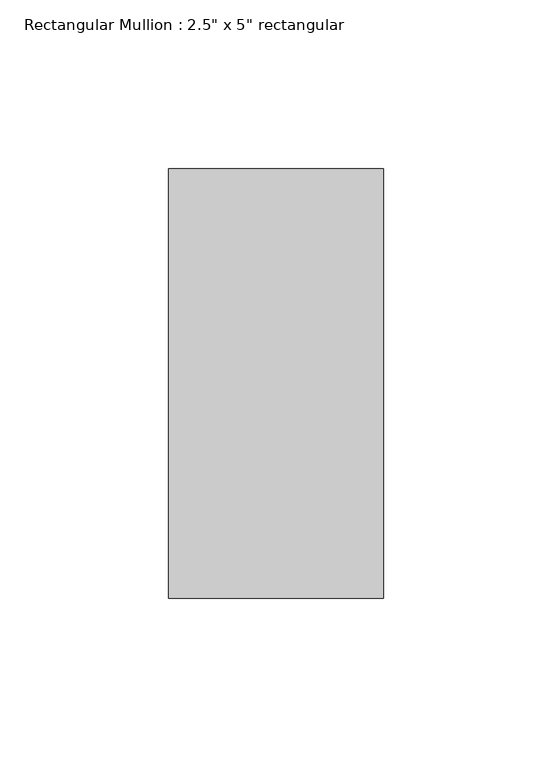
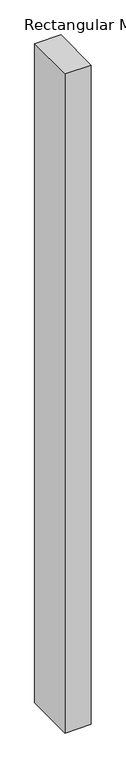
"""IFC4 building model written with IfcOpenShell, lengths in millimetres: member geometry."""

from ifc_helpers import new_model, si_unit, frame, origin, place, context, project, spatial, polyline, outline, extrude, source, transform, mapped, element, save


def member_4cef4026(model_context):
    return source(origin(), model_context, "Body", "SweptSolid", [
        extrude(outline(polyline([(0.0, 63.5), (0.0, -63.5), (-63.5, -63.5), (-63.5, 63.5), (0.0, 63.5)])), frame((0.0, 0.0, -1687.096911), z_axis=(0.0, 0.0, 1.0), x_axis=(1.0, 0.0, 0.0)), (0.0, 0.0, 1.0), 1687.096911),
    ])


if __name__ == "__main__":
    model = new_model("IFC4")
    model_context = context("Model", 3, world=origin())
    ifc_project = project(units=[si_unit("LENGTHUNIT", "METRE", prefix="MILLI")], contexts=[model_context])
    site = spatial("IfcSite", under=ifc_project)
    building = spatial("IfcBuilding", under=site)
    placement = place(None, origin())
    member_shape = member_4cef4026(model_context)
    element("IfcMember", 1, ObjectType="Rectangular Mullion : 2.5\" x 5\" rectangular", at=placement, inside=building, context=model_context, shape_type="MappedRepresentation", body=[
        mapped(member_shape, transform((0.0, 0.0, 0.0), x_axis=(1.0, 0.0, 0.0), y_axis=(0.0, 1.0, 0.0), z_axis=(0.0, 0.0, 1.0))),
    ])
    save(model, "model.ifc")

# Revit data of these elements
# Type "Rectangular Mullion : 2.5\" x 5\" rectangular"
#   built-in parameter 1007304 = 0.416667 (stored number, unit not read)
#   built-in parameter 1007301 = 0.104167 (stored number, unit not read)
#   built-in parameter 1007300 = 0.104167 (stored number, unit not read)
# Element 1 (IfcMember, "Rectangular Mullion : 2.5\" x 5\" rectangular")
#   Materials on its faces: "Aluminum"
# Materials
#   "Aluminum": class "Metal", colour RGB 247 247 247, transparency 0, Description = "Aluminum 6061", Cost = 0
